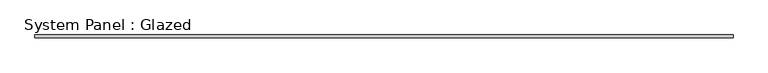
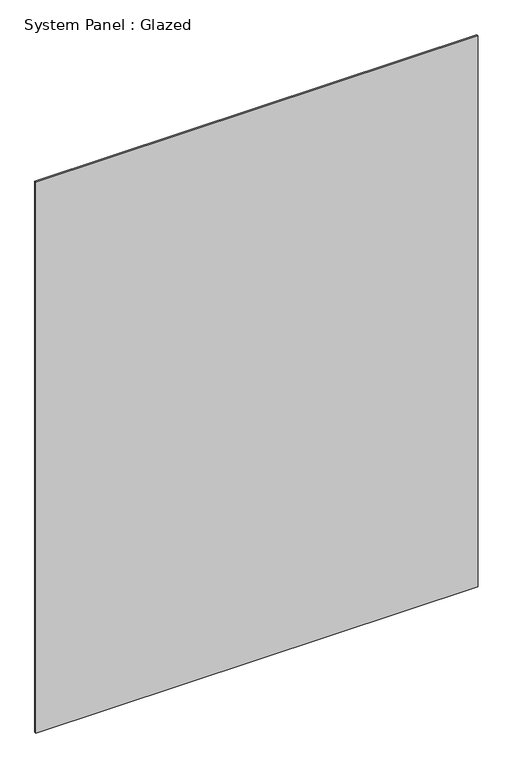
"""IFC4 building model written with IfcOpenShell, lengths in millimetres: plate geometry, System Panel : Glazed."""

from ifc_helpers import new_model, si_unit, origin, origin_with_axes, place, context, project, spatial, polyline, outline, extrude, source, transform, mapped, element, save


def system_panel_glazed_816a57b3(model_context):
    return source(origin(), model_context, "Body", "SweptSolid", [
        extrude(outline(polyline([(708.3333334, 34.0), (-708.3333334, 34.0), (-708.3333334, 40.0), (708.3333334, 40.0), (708.3333334, 34.0)])), origin_with_axes(), (0.0, 0.0, 1.0), 1865.4113705),
    ])


if __name__ == "__main__":
    model = new_model("IFC4")
    model_context = context("Model", 3, world=origin())
    ifc_project = project(units=[si_unit("LENGTHUNIT", "METRE", prefix="MILLI")], contexts=[model_context])
    site = spatial("IfcSite", under=ifc_project)
    building = spatial("IfcBuilding", under=site)
    placement = place(None, origin())
    system_panel_glazed_shape = system_panel_glazed_816a57b3(model_context)
    element("IfcPlate", 1, ObjectType="System Panel : Glazed", at=placement, inside=building, context=model_context, shape_type="MappedRepresentation", body=[
        mapped(system_panel_glazed_shape, transform((0.0, 0.0, 0.0), x_axis=(1.0, 0.0, 0.0), y_axis=(0.0, 1.0, 0.0), z_axis=(0.0, 0.0, 1.0))),
    ])
    save(model, "model.ifc")

# Revit data of these elements
# Type "System Panel : Glazed"
#   Construction Type Id = "GSP4R"
#   Analytic Construction = "1/8 in Pilkington single glazing"
#   Visual Light Transmittance = 0.9
#   Solar Heat Gain Coefficient = 0.86
#   Heat Transfer Coefficient (U) = 6.7069 W/(m²·K)
#   Define Thermal Properties by = 1
# Element 1 (IfcPlate, "System Panel : Glazed")
#   Materials on its faces: "Default New Material(6)"
# Materials
#   "Default New Material(6)": class "Generic", colour RGB 191 25 25, transparency 0.9, Cost = 0
